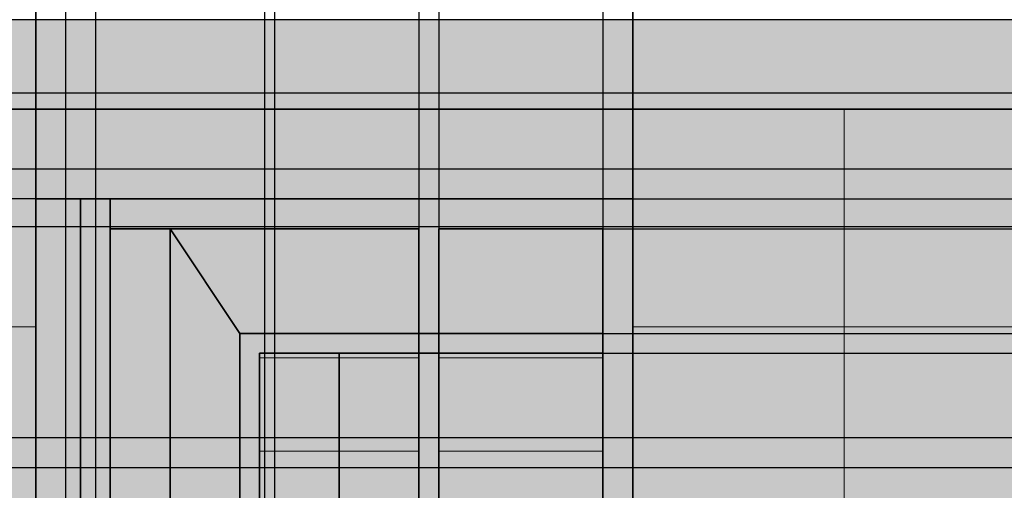
# Model space of a CAD drawing. Units: inches. Extents: x 148 to 1080, y 89 to 707.
# Tile 5 of 12: x 272 to 470, y 273 to 368. Entities that reach past the tile are written whole.
import ezdxf

# ---------------------------------------------------------------- set-up
doc = ezdxf.new("R2010")
doc.units = ezdxf.units.IN
doc.header["$MEASUREMENT"] = 0
for name, color, linetype, lineweight in [('A-ANNO-DIMS', 2, 'Continuous', 18), ('A-ELEV', 7, 'Continuous', 35), ('A-ELEV-PATT', 8, 'Continuous', 13)]:
    doc.layers.add(name, color=color, linetype=linetype, lineweight=lineweight)
doc.styles.get("Standard").update_dxf_attribs({"font": 'arial.ttf'})
doc.dimstyles.get("Standard").update_dxf_attribs({"dimtxt": 6, "dimasz": 0.18, "dimexe": 0.18, "dimexo": 0.0625, "dimgap": 0.09, "dimtad": 0, "dimtih": 1, "dimtoh": 1, "dimdec": 0, "dimzin": 0, "dimdsep": 46, "dimlunit": 3, "dimtxsty": 'Standard', "dimcen": 0.09, "dimadec": 0, "dimazin": 0, "dimtfac": 1, "dimtdec": 0, "dimtofl": 0, "dimtmove": 0, "dimatfit": 3, "dimfxl": 1, "dimtolj": 1, "dimtzin": 0, "dimarcsym": 0})

# ---------------------------------------------------------------- blocks, each defined once
blk = doc.blocks.new('*D1')
at = {"layer": 'A-ANNO-DIMS', "color": 0, "lineweight": -2, "transparency": 16777216}
for p, q in [((215.02, 662.01), (215.02, 703.28)), ((215.2, 703.1), (604.32, 703.1)), ((1006.77, 703.1), (617.65, 703.1)), ((1006.95, 338.01), (1006.95, 703.28))]:
    blk.add_line(p, q, dxfattribs=at)
at = {"layer": 'A-ANNO-DIMS', "color": 0, "transparency": 16777216}
for points in [[(215.2, 703.13), (215.2, 703.07), (215.02, 703.1)], [(1006.77, 703.13), (1006.77, 703.07), (1006.95, 703.1)]]:
    blk.add_solid(points, dxfattribs=at)
at = {"layer": 'Defpoints', "color": 0, "transparency": 16777216}
for p in [(1006.95, 703.1), (215.02, 661.95), (1006.95, 337.95)]:
    blk.add_point(p, dxfattribs=at)
at = {"layer": 'A-ANNO-DIMS', "color": 0, "transparency": 16777216, "insert": (610.98, 703.1), "char_height": 6, "attachment_point": 5}
blk.add_mtext('\\A1;792', dxfattribs=at)
blk = doc.blocks.new('*D27')
at = {"layer": 'A-ANNO-DIMS', "color": 0, "lineweight": -2, "transparency": 16777216}
for p, q in [((275.02, 332.01), (275.02, 703.28)), ((275.2, 703.1), (328.59, 703.1)), ((394.84, 703.1), (341.45, 703.1)), ((395.02, 332.01), (395.02, 703.28))]:
    blk.add_line(p, q, dxfattribs=at)
at = {"layer": 'A-ANNO-DIMS', "color": 0, "transparency": 16777216}
for points in [[(275.2, 703.13), (275.2, 703.07), (275.02, 703.1)], [(394.84, 703.13), (394.84, 703.07), (395.02, 703.1)]]:
    blk.add_solid(points, dxfattribs=at)
at = {"layer": 'Defpoints', "color": 0, "transparency": 16777216}
for p in [(395.02, 703.1), (275.02, 331.95), (395.02, 331.95)]:
    blk.add_point(p, dxfattribs=at)
at = {"layer": 'A-ANNO-DIMS', "color": 0, "transparency": 16777216, "insert": (335.02, 703.1), "char_height": 6, "attachment_point": 5}
blk.add_mtext('\\A1;120', dxfattribs=at)
blk = doc.blocks.new('*D28')
at = {"layer": 'A-ANNO-DIMS', "color": 0, "lineweight": -2, "transparency": 16777216}
for p, q in [((274.96, 331.95), (160.42, 331.95)), ((160.6, 331.77), (160.6, 251.1)), ((160.6, 164.13), (160.6, 244.79)), ((274.96, 163.95), (160.42, 163.95))]:
    blk.add_line(p, q, dxfattribs=at)
at = {"layer": 'A-ANNO-DIMS', "color": 0, "transparency": 16777216}
for points in [[(160.57, 331.77), (160.63, 331.77), (160.6, 331.95)], [(160.57, 164.13), (160.63, 164.13), (160.6, 163.95)]]:
    blk.add_solid(points, dxfattribs=at)
at = {"layer": 'Defpoints', "color": 0, "transparency": 16777216}
for p in [(160.6, 331.95), (275.02, 331.95), (275.02, 163.95)]:
    blk.add_point(p, dxfattribs=at)
at = {"layer": 'A-ANNO-DIMS', "color": 0, "transparency": 16777216, "insert": (160.6, 247.95), "char_height": 6, "attachment_point": 5}
blk.add_mtext('\\A1;168', dxfattribs=at)
blk = doc.blocks.new('*D34')
at = {"layer": 'A-ANNO-DIMS', "color": 0, "lineweight": -2, "transparency": 16777216}
for p, q in [((574.96, 283.95), (160.42, 283.95)), ((160.6, 283.77), (160.6, 212.1)), ((160.6, 134.13), (160.6, 205.79)), ((574.96, 133.95), (160.42, 133.95))]:
    blk.add_line(p, q, dxfattribs=at)
at = {"layer": 'A-ANNO-DIMS', "color": 0, "transparency": 16777216}
for points in [[(160.57, 283.77), (160.63, 283.77), (160.6, 283.95)], [(160.57, 134.13), (160.63, 134.13), (160.6, 133.95)]]:
    blk.add_solid(points, dxfattribs=at)
at = {"layer": 'Defpoints', "color": 0, "transparency": 16777216}
for p in [(575.02, 283.95), (160.6, 133.95), (575.02, 133.95)]:
    blk.add_point(p, dxfattribs=at)
at = {"layer": 'A-ANNO-DIMS', "color": 0, "transparency": 16777216, "insert": (160.6, 208.95), "char_height": 6, "attachment_point": 5}
blk.add_mtext('\\A1;150', dxfattribs=at)
blk = doc.blocks.new('*D39')
at = {"layer": 'A-ANNO-DIMS', "color": 0, "lineweight": -2, "transparency": 16777216}
for p, q in [((946.89, 337.95), (160.42, 337.95)), ((160.6, 337.77), (160.6, 311.1)), ((160.6, 278.13), (160.6, 304.79)), ((946.89, 277.95), (160.42, 277.95))]:
    blk.add_line(p, q, dxfattribs=at)
at = {"layer": 'A-ANNO-DIMS', "color": 0, "transparency": 16777216}
for points in [[(160.57, 337.77), (160.63, 337.77), (160.6, 337.95)], [(160.57, 278.13), (160.63, 278.13), (160.6, 277.95)]]:
    blk.add_solid(points, dxfattribs=at)
at = {"layer": 'Defpoints', "color": 0, "transparency": 16777216}
for p in [(160.6, 337.95), (946.95, 337.95), (946.95, 277.95)]:
    blk.add_point(p, dxfattribs=at)
at = {"layer": 'A-ANNO-DIMS', "color": 0, "transparency": 16777216, "insert": (160.6, 307.95), "char_height": 6, "attachment_point": 5}
blk.add_mtext('\\A1;60', dxfattribs=at)
blk = doc.blocks.new('*D42')
at = {"layer": 'A-ANNO-DIMS', "color": 0, "lineweight": -2, "transparency": 16777216}
for p, q in [((772.96, 367.95), (160.42, 367.95)), ((160.6, 367.77), (160.6, 350.31)), ((160.6, 326.54), (160.6, 344)), ((718.96, 326.36), (160.42, 326.36))]:
    blk.add_line(p, q, dxfattribs=at)
at = {"layer": 'A-ANNO-DIMS', "color": 0, "transparency": 16777216}
for points in [[(160.57, 367.77), (160.63, 367.77), (160.6, 367.95)], [(160.57, 326.54), (160.63, 326.54), (160.6, 326.36)]]:
    blk.add_solid(points, dxfattribs=at)
at = {"layer": 'Defpoints', "color": 0, "transparency": 16777216}
for p in [(773.02, 367.95), (160.6, 326.36), (719.02, 326.36)]:
    blk.add_point(p, dxfattribs=at)
at = {"layer": 'A-ANNO-DIMS', "color": 0, "transparency": 16777216, "insert": (160.6, 347.16), "char_height": 6, "attachment_point": 5}
blk.add_mtext('\\A1;41.584', dxfattribs=at)
blk = doc.blocks.new('*D49')
at = {"layer": 'A-ANNO-DIMS', "color": 0, "lineweight": -2, "transparency": 16777216}
for p, q in [((628.11, 353.2), (160.42, 353.2)), ((160.6, 353.02), (160.6, 348.73)), ((160.6, 338.13), (160.6, 342.42)), ((682.96, 337.95), (160.42, 337.95))]:
    blk.add_line(p, q, dxfattribs=at)
at = {"layer": 'A-ANNO-DIMS', "color": 0, "transparency": 16777216}
for points in [[(160.57, 353.02), (160.63, 353.02), (160.6, 353.2)], [(160.57, 338.13), (160.63, 338.13), (160.6, 337.95)]]:
    blk.add_solid(points, dxfattribs=at)
at = {"layer": 'Defpoints', "color": 0, "transparency": 16777216}
for p in [(628.17, 353.2), (160.6, 337.95), (683.02, 337.95)]:
    blk.add_point(p, dxfattribs=at)
at = {"layer": 'A-ANNO-DIMS', "color": 0, "transparency": 16777216, "insert": (160.6, 345.57), "char_height": 6, "attachment_point": 5}
blk.add_mtext('\\A1;15.248', dxfattribs=at)
blk = doc.blocks.new('*D76')
at = {"layer": 'A-ANNO-DIMS', "color": 0, "lineweight": -2, "transparency": 16777216}
for p, q in [((389.08, 300.95), (1064.5, 300.95)), ((1064.32, 300.77), (1064.32, 286.06)), ((1064.32, 265.05), (1064.32, 279.75)), ((389.08, 264.87), (1064.5, 264.87))]:
    blk.add_line(p, q, dxfattribs=at)
at = {"layer": 'A-ANNO-DIMS', "color": 0, "transparency": 16777216}
for points in [[(1064.29, 300.77), (1064.35, 300.77), (1064.32, 300.95)], [(1064.29, 265.05), (1064.35, 265.05), (1064.32, 264.87)]]:
    blk.add_solid(points, dxfattribs=at)
at = {"layer": 'Defpoints', "color": 0, "transparency": 16777216}
for p in [(389.02, 300.95), (1064.32, 300.95), (389.02, 264.87)]:
    blk.add_point(p, dxfattribs=at)
at = {"layer": 'A-ANNO-DIMS', "color": 0, "transparency": 16777216, "insert": (1064.32, 282.91), "char_height": 6, "attachment_point": 5}
blk.add_mtext('\\A1;36.08', dxfattribs=at)
blk = doc.blocks.new('*D77')
at = {"layer": 'A-ANNO-DIMS', "color": 0, "lineweight": -2, "transparency": 16777216}
for p, q in [((389.08, 304.95), (1064.5, 304.95)), ((1064.32, 304.95), (1064.32, 305.13)), ((1064.32, 305.13), (1064.5, 305.13)), ((1064.32, 301.13), (1064.32, 304.77)), ((389.08, 300.95), (1064.5, 300.95))]:
    blk.add_line(p, q, dxfattribs=at)
at = {"layer": 'A-ANNO-DIMS', "color": 0, "transparency": 16777216}
for points in [[(1064.29, 304.77), (1064.35, 304.77), (1064.32, 304.95)], [(1064.29, 301.13), (1064.35, 301.13), (1064.32, 300.95)]]:
    blk.add_solid(points, dxfattribs=at)
at = {"layer": 'Defpoints', "color": 0, "transparency": 16777216}
for p in [(389.02, 304.95), (1064.32, 304.95), (389.02, 300.95)]:
    blk.add_point(p, dxfattribs=at)
at = {"layer": 'A-ANNO-DIMS', "color": 0, "transparency": 16777216, "insert": (1072.5, 305.13), "char_height": 6, "attachment_point": 5}
blk.add_mtext('\\A1;4.00', dxfattribs=at)
blk = doc.blocks.new('*D78')
at = {"layer": 'A-ANNO-DIMS', "color": 0, "lineweight": -2, "transparency": 16777216}
for p, q in [((389.08, 325.95), (1064.5, 325.95)), ((1064.32, 325.77), (1064.32, 318.6)), ((1064.32, 305.13), (1064.32, 312.29)), ((389.08, 304.95), (1064.5, 304.95))]:
    blk.add_line(p, q, dxfattribs=at)
at = {"layer": 'A-ANNO-DIMS', "color": 0, "transparency": 16777216}
for points in [[(1064.29, 325.77), (1064.35, 325.77), (1064.32, 325.95)], [(1064.29, 305.13), (1064.35, 305.13), (1064.32, 304.95)]]:
    blk.add_solid(points, dxfattribs=at)
at = {"layer": 'Defpoints', "color": 0, "transparency": 16777216}
for p in [(389.02, 325.95), (1064.32, 325.95), (389.02, 304.95)]:
    blk.add_point(p, dxfattribs=at)
at = {"layer": 'A-ANNO-DIMS', "color": 0, "transparency": 16777216, "insert": (1064.32, 315.45), "char_height": 6, "attachment_point": 5}
blk.add_mtext('\\A1;21.00', dxfattribs=at)
blk = doc.blocks.new('*D79')
at = {"layer": 'A-ANNO-DIMS', "color": 0, "lineweight": -2, "transparency": 16777216}
for p, q in [((395.08, 331.95), (1064.5, 331.95)), ((1064.32, 331.95), (1064.32, 332.13)), ((1064.32, 332.13), (1064.5, 332.13)), ((1064.32, 326.13), (1064.32, 331.77)), ((389.08, 325.95), (1064.5, 325.95))]:
    blk.add_line(p, q, dxfattribs=at)
at = {"layer": 'A-ANNO-DIMS', "color": 0, "transparency": 16777216}
for points in [[(1064.29, 331.77), (1064.35, 331.77), (1064.32, 331.95)], [(1064.29, 326.13), (1064.35, 326.13), (1064.32, 325.95)]]:
    blk.add_solid(points, dxfattribs=at)
at = {"layer": 'Defpoints', "color": 0, "transparency": 16777216}
for p in [(395.02, 331.95), (1064.32, 331.95), (389.02, 325.95)]:
    blk.add_point(p, dxfattribs=at)
at = {"layer": 'A-ANNO-DIMS', "color": 0, "transparency": 16777216, "insert": (1072.39, 332.13), "char_height": 6, "attachment_point": 5}
blk.add_mtext('\\A1;6.00', dxfattribs=at)
blk = doc.blocks.new('*D82')
at = {"layer": 'A-ANNO-DIMS', "color": 0, "lineweight": -2, "transparency": 16777216}
for p, q in [((275.02, 400.88), (275.02, 92.62)), ((281.02, 400.88), (281.02, 92.62)), ((275.2, 92.8), (280.84, 92.8)), ((281.02, 92.8), (281.2, 92.8))]:
    blk.add_line(p, q, dxfattribs=at)
at = {"layer": 'A-ANNO-DIMS', "color": 0, "transparency": 16777216}
for points in [[(275.2, 92.83), (275.2, 92.77), (275.02, 92.8)], [(280.84, 92.83), (280.84, 92.77), (281.02, 92.8)]]:
    blk.add_solid(points, dxfattribs=at)
at = {"layer": 'Defpoints', "color": 0, "transparency": 16777216}
for p in [(275.02, 400.95), (281.02, 400.95), (281.02, 92.8)]:
    blk.add_point(p, dxfattribs=at)
at = {"layer": 'A-ANNO-DIMS', "color": 0, "transparency": 16777216, "insert": (289.09, 92.8), "char_height": 6, "attachment_point": 5}
blk.add_mtext('\\A1;6.00', dxfattribs=at)
blk = doc.blocks.new('*D83')
at = {"layer": 'A-ANNO-DIMS', "color": 0, "lineweight": -2, "transparency": 16777216}
for p, q in [((281.02, 400.88), (281.02, 92.62)), ((287.02, 400.88), (287.02, 92.62)), ((281.2, 92.8), (286.84, 92.8)), ((287.02, 92.8), (287.2, 92.8))]:
    blk.add_line(p, q, dxfattribs=at)
at = {"layer": 'A-ANNO-DIMS', "color": 0, "transparency": 16777216}
for points in [[(281.2, 92.83), (281.2, 92.77), (281.02, 92.8)], [(286.84, 92.83), (286.84, 92.77), (287.02, 92.8)]]:
    blk.add_solid(points, dxfattribs=at)
at = {"layer": 'Defpoints', "color": 0, "transparency": 16777216}
for p in [(281.02, 400.95), (287.02, 400.95), (287.02, 92.8)]:
    blk.add_point(p, dxfattribs=at)
at = {"layer": 'A-ANNO-DIMS', "color": 0, "transparency": 16777216, "insert": (295.09, 92.8), "char_height": 6, "attachment_point": 5}
blk.add_mtext('\\A1;6.00', dxfattribs=at)
blk = doc.blocks.new('*D84')
at = {"layer": 'A-ANNO-DIMS', "color": 0, "lineweight": -2, "transparency": 16777216}
for p, q in [((321.02, 529.88), (321.02, 92.62)), ((287.02, 400.88), (287.02, 92.62)), ((287.2, 92.8), (293.82, 92.8)), ((320.84, 92.8), (314.22, 92.8))]:
    blk.add_line(p, q, dxfattribs=at)
at = {"layer": 'A-ANNO-DIMS', "color": 0, "transparency": 16777216}
for points in [[(287.2, 92.83), (287.2, 92.77), (287.02, 92.8)], [(320.84, 92.83), (320.84, 92.77), (321.02, 92.8)]]:
    blk.add_solid(points, dxfattribs=at)
at = {"layer": 'Defpoints', "color": 0, "transparency": 16777216}
for p in [(321.02, 529.95), (287.02, 400.95), (321.02, 92.8)]:
    blk.add_point(p, dxfattribs=at)
at = {"layer": 'A-ANNO-DIMS', "color": 0, "transparency": 16777216, "insert": (304.02, 92.8), "char_height": 6, "attachment_point": 5}
blk.add_mtext('\\A1;34.00', dxfattribs=at)
blk = doc.blocks.new('*D85')
at = {"layer": 'A-ANNO-DIMS', "color": 0, "lineweight": -2, "transparency": 16777216}
for p, q in [((321.02, 529.88), (321.02, 92.62)), ((323.02, 400.88), (323.02, 92.62)), ((321.2, 92.8), (322.84, 92.8)), ((323.02, 92.8), (323.2, 92.8))]:
    blk.add_line(p, q, dxfattribs=at)
at = {"layer": 'A-ANNO-DIMS', "color": 0, "transparency": 16777216}
for points in [[(321.2, 92.83), (321.2, 92.77), (321.02, 92.8)], [(322.84, 92.83), (322.84, 92.77), (323.02, 92.8)]]:
    blk.add_solid(points, dxfattribs=at)
at = {"layer": 'Defpoints', "color": 0, "transparency": 16777216}
for p in [(321.02, 529.95), (323.02, 400.95), (323.02, 92.8)]:
    blk.add_point(p, dxfattribs=at)
at = {"layer": 'A-ANNO-DIMS', "color": 0, "transparency": 16777216, "insert": (331.12, 92.8), "char_height": 6, "attachment_point": 5}
blk.add_mtext('\\A1;2.00', dxfattribs=at)
blk = doc.blocks.new('*D86')
at = {"layer": 'A-ANNO-DIMS', "color": 0, "lineweight": -2, "transparency": 16777216}
for p, q in [((323.02, 400.88), (323.02, 92.62)), ((352.02, 400.88), (352.02, 92.62)), ((323.2, 92.8), (327.27, 92.8)), ((351.84, 92.8), (347.77, 92.8))]:
    blk.add_line(p, q, dxfattribs=at)
at = {"layer": 'A-ANNO-DIMS', "color": 0, "transparency": 16777216}
for points in [[(323.2, 92.83), (323.2, 92.77), (323.02, 92.8)], [(351.84, 92.83), (351.84, 92.77), (352.02, 92.8)]]:
    blk.add_solid(points, dxfattribs=at)
at = {"layer": 'Defpoints', "color": 0, "transparency": 16777216}
for p in [(323.02, 400.95), (352.02, 400.95), (352.02, 92.8)]:
    blk.add_point(p, dxfattribs=at)
at = {"layer": 'A-ANNO-DIMS', "color": 0, "transparency": 16777216, "insert": (337.52, 92.8), "char_height": 6, "attachment_point": 5}
blk.add_mtext('\\A1;29.00', dxfattribs=at)
blk = doc.blocks.new('*D87')
at = {"layer": 'A-ANNO-DIMS', "color": 0, "lineweight": -2, "transparency": 16777216}
for p, q in [((352.02, 400.88), (352.02, 92.62)), ((356.02, 400.88), (356.02, 92.62)), ((352.2, 92.8), (355.84, 92.8)), ((356.02, 92.8), (356.2, 92.8))]:
    blk.add_line(p, q, dxfattribs=at)
at = {"layer": 'A-ANNO-DIMS', "color": 0, "transparency": 16777216}
for points in [[(352.2, 92.83), (352.2, 92.77), (352.02, 92.8)], [(355.84, 92.83), (355.84, 92.77), (356.02, 92.8)]]:
    blk.add_solid(points, dxfattribs=at)
at = {"layer": 'Defpoints', "color": 0, "transparency": 16777216}
for p in [(352.02, 400.95), (356.02, 400.95), (356.02, 92.8)]:
    blk.add_point(p, dxfattribs=at)
at = {"layer": 'A-ANNO-DIMS', "color": 0, "transparency": 16777216, "insert": (364.19, 92.8), "char_height": 6, "attachment_point": 5}
blk.add_mtext('\\A1;4.00', dxfattribs=at)
blk = doc.blocks.new('*D88')
at = {"layer": 'A-ANNO-DIMS', "color": 0, "lineweight": -2, "transparency": 16777216}
for p, q in [((356.02, 400.88), (356.02, 92.62)), ((389.02, 400.88), (389.02, 92.62)), ((356.2, 92.8), (362.32, 92.8)), ((388.84, 92.8), (382.72, 92.8))]:
    blk.add_line(p, q, dxfattribs=at)
at = {"layer": 'A-ANNO-DIMS', "color": 0, "transparency": 16777216}
for points in [[(356.2, 92.83), (356.2, 92.77), (356.02, 92.8)], [(388.84, 92.83), (388.84, 92.77), (389.02, 92.8)]]:
    blk.add_solid(points, dxfattribs=at)
at = {"layer": 'Defpoints', "color": 0, "transparency": 16777216}
for p in [(356.02, 400.95), (389.02, 400.95), (389.02, 92.8)]:
    blk.add_point(p, dxfattribs=at)
at = {"layer": 'A-ANNO-DIMS', "color": 0, "transparency": 16777216, "insert": (372.52, 92.8), "char_height": 6, "attachment_point": 5}
blk.add_mtext('\\A1;33.00', dxfattribs=at)
blk = doc.blocks.new('*D89')
at = {"layer": 'A-ANNO-DIMS', "color": 0, "lineweight": -2, "transparency": 16777216}
for p, q in [((389.02, 400.88), (389.02, 92.62)), ((395.02, 400.88), (395.02, 92.62)), ((389.2, 92.8), (394.84, 92.8)), ((395.02, 92.8), (395.2, 92.8))]:
    blk.add_line(p, q, dxfattribs=at)
at = {"layer": 'A-ANNO-DIMS', "color": 0, "transparency": 16777216}
for points in [[(389.2, 92.83), (389.2, 92.77), (389.02, 92.8)], [(394.84, 92.83), (394.84, 92.77), (395.02, 92.8)]]:
    blk.add_solid(points, dxfattribs=at)
at = {"layer": 'Defpoints', "color": 0, "transparency": 16777216}
for p in [(389.02, 400.95), (395.02, 400.95), (395.02, 92.8)]:
    blk.add_point(p, dxfattribs=at)
at = {"layer": 'A-ANNO-DIMS', "color": 0, "transparency": 16777216, "insert": (403.09, 92.8), "char_height": 6, "attachment_point": 5}
blk.add_mtext('\\A1;6.00', dxfattribs=at)

msp = doc.modelspace()

# ---------------------------------------------------------------- hatches: boundary and pattern name
at = {"layer": 'A-ELEV-PATT'}
h = msp.add_hatch(color=256, dxfattribs=at)
h.dxf.hatch_style = 1
h.paths.add_polyline_path([(622.6005, 631.9474), (611.0199, 631.9474), (215.0199, 631.9474), (251.0199, 542.9352), (251.0199, 601.9474), (527.0199, 601.9474), (527.0199, 541.9474), (598.6005, 541.9474)])
h.paths.add_polyline_path([(558.5775, 608.9493, -1), (552.5775, 608.9493, -1)], flags=16)
h.paths.add_polyline_path([(586.7589, 556.0652, -1), (580.7589, 556.0652, -1)], flags=16)
h.paths.add_polyline_path([(635.0199, 631.9474), (622.6005, 631.9474), (598.6005, 541.9474), (611.0199, 541.9474)])
h.paths.add_polyline_path([(773.0199, 367.9474), (215.0199, 367.9474), (251.0199, 337.9474), (251.0199, 349.9474), (527.0199, 349.9474), (527.0199, 337.9474), (734.0628, 337.9474)])
h.paths.add_polyline_path([(631.1736, 353.1958, -1), (625.1736, 353.1958, -1)], flags=16)
h.paths.add_polyline_path([(729.9419, 354.8591, -1), (723.9419, 354.8591, -1)], flags=16)
h = msp.add_hatch(color=256, dxfattribs=at)
h.dxf.hatch_style = 1
h.paths.add_polyline_path([(395.0199, 349.9474), (275.0199, 349.9474), (275.0199, 331.9474), (395.0199, 331.9474)])
h.paths.add_polyline_path([(284.0199, 331.9474), (275.0199, 331.9474), (275.0199, 163.9474), (284.0199, 163.9474)])
h.paths.add_polyline_path([(395.0199, 601.9474), (251.0199, 601.9474), (251.0199, 589.9474), (395.0199, 589.9474)])
h = msp.add_hatch(color=256, dxfattribs=at)
h.dxf.hatch_style = 1
h.paths.add_polyline_path([(527.0199, 349.9474), (395.0199, 349.9474), (395.0199, 271.2774), (527.0199, 272.3839)])
h.paths.add_polyline_path([(275.0199, 349.9474), (251.0199, 349.9474), (251.0199, 270.0704), (275.0199, 270.2716)])
h.paths.add_polyline_path([(743.0199, 337.9474), (734.0628, 337.9474), (719.0199, 326.3632), (719.0199, 277.9474), (743.0199, 277.9474)])
h.paths.add_polyline_path([(743.0199, 277.9474), (719.0199, 277.9474), (719.0199, 133.9474), (743.0199, 133.9474)])
h.paths.add_polyline_path([(734.0628, 337.9474), (719.0199, 337.9474), (719.0199, 326.3632)])
h = msp.add_hatch(dxfattribs=at)
h.set_pattern_fill('ANSI37', color=256, scale=350, angle=135)
h.paths.add_polyline_path([(527.0199, 349.9474), (395.0199, 349.9474), (395.0199, 163.9474), (275.0199, 163.9474), (275.0199, 349.9474), (251.0199, 349.9474), (251.0199, 133.9474), (527.0199, 133.9474)])
h = msp.add_hatch(color=256, dxfattribs=at)
h.dxf.hatch_style = 1
h.paths.add_polyline_path([(290.0199, 331.9474), (284.0199, 331.9474), (284.0199, 163.9474), (395.0199, 163.9474), (395.0199, 331.9474), (290.0199, 331.9474), (290.0199, 325.9474), (352.0199, 325.9474), (352.0199, 304.9474), (356.0199, 304.9474), (356.0199, 325.9474), (389.0199, 325.9474), (389.0199, 169.9474), (290.0199, 169.9474)])
h.paths.add_polyline_path([(356.0199, 300.9474), (352.0199, 300.9474), (352.0199, 169.9474), (356.0199, 169.9474)], flags=17)
h.paths.add_polyline_path([(356.0199, 304.9474), (352.0199, 304.9474), (352.0199, 300.9474), (356.0199, 300.9474)], flags=17)
h = msp.add_hatch(color=256, dxfattribs=at)
h.dxf.hatch_style = 1
h.paths.add_polyline_path([(389.0199, 300.9474), (356.0199, 300.9474), (356.0199, 264.8696), (389.0199, 264.8696)])
h.paths.add_polyline_path([(389.0199, 325.9474), (356.0199, 325.9474), (356.0199, 304.9474), (389.0199, 304.9474)])
h.paths.add_polyline_path([(352.0199, 325.9474), (302.0199, 325.9474), (316.0199, 304.9474), (352.0199, 304.9474)])
h.paths.add_polyline_path([(316.0199, 304.9474), (302.0199, 325.9474), (302.0199, 169.9474), (316.0199, 169.9474)])
h.paths.add_polyline_path([(302.0199, 325.9474), (290.0199, 325.9474), (290.0199, 222.3199), (302.0199, 206.8913)])
h.paths.add_polyline_path([(320.0199, 300.9474), (352.0199, 300.9474), (352.0199, 304.9474), (316.0199, 304.9474), (316.0199, 169.9474), (320.0199, 169.9474)])
h.paths.add_polyline_path([(336.0199, 300.9474), (320.0199, 300.9474), (320.0199, 264.8696), (336.0199, 264.8696)], flags=17)
h.paths.add_polyline_path([(352.0199, 300.9474), (336.0199, 300.9474), (336.0199, 264.8696), (352.0199, 264.8696)])
h.paths.add_polyline_path([(389.0199, 304.9474), (356.0199, 304.9474), (356.0199, 300.9474), (389.0199, 300.9474)])
h.paths.add_polyline_path([(389.0199, 192.8696), (356.0199, 192.8696), (356.0199, 169.9474), (389.0199, 169.9474)])
h.paths.add_polyline_path([(389.0199, 216.8696), (356.0199, 216.8696), (356.0199, 192.8696), (389.0199, 192.8696)])
h.paths.add_polyline_path([(389.0199, 240.8696), (356.0199, 240.8696), (356.0199, 216.8696), (389.0199, 216.8696)])
h.paths.add_polyline_path([(389.0199, 264.8696), (356.0199, 264.8696), (356.0199, 240.8696), (389.0199, 240.8696)])
h.paths.add_polyline_path([(352.0199, 264.8696), (336.0199, 264.8696), (336.0199, 240.8696), (352.0199, 240.8696)])
h.paths.add_polyline_path([(336.0199, 264.8696), (320.0199, 264.8696), (320.0199, 240.8696), (336.0199, 240.8696)], flags=17)
h.paths.add_polyline_path([(336.0199, 240.8696), (320.0199, 240.8696), (320.0199, 216.8696), (336.0199, 216.8696)], flags=17)
h.paths.add_polyline_path([(352.0199, 240.8696), (336.0199, 240.8696), (336.0199, 216.8696), (352.0199, 216.8696)])
h.paths.add_polyline_path([(352.0199, 216.8696), (336.0199, 216.8696), (336.0199, 192.8696), (352.0199, 192.8696)])
h.paths.add_polyline_path([(336.0199, 216.8696), (320.0199, 216.8696), (320.0199, 192.8696), (336.0199, 192.8696)], flags=17)
h.paths.add_polyline_path([(336.0199, 192.8696), (320.0199, 192.8696), (320.0199, 169.9474), (336.0199, 169.9474)], flags=17)
h.paths.add_polyline_path([(352.0199, 192.8696), (336.0199, 192.8696), (336.0199, 169.9474), (352.0199, 169.9474)])
h = msp.add_hatch(dxfattribs=at)
h.set_pattern_fill('ANSI31', color=256, scale=150, angle=135)
h.paths.add_polyline_path([(389.0199, 192.8696), (356.0199, 192.8696), (356.0199, 169.9474), (389.0199, 169.9474)])
h.paths.add_polyline_path([(389.0199, 240.8696), (356.0199, 240.8696), (356.0199, 216.8696), (389.0199, 216.8696)])
h.paths.add_polyline_path([(389.0199, 216.8696), (356.0199, 216.8696), (356.0199, 192.8696), (389.0199, 192.8696)])
h.paths.add_polyline_path([(389.0199, 264.8696), (356.0199, 264.8696), (356.0199, 240.8696), (389.0199, 240.8696)])
h.paths.add_polyline_path([(389.0199, 300.9474), (356.0199, 300.9474), (356.0199, 264.8696), (389.0199, 264.8696)])
h.paths.add_polyline_path([(352.0199, 300.9474), (336.0199, 300.9474), (336.0199, 264.8696), (352.0199, 264.8696)])
h.paths.add_polyline_path([(336.0199, 300.9474), (320.0199, 300.9474), (320.0199, 264.8696), (336.0199, 264.8696)])
h.paths.add_polyline_path([(336.0199, 264.8696), (320.0199, 264.8696), (320.0199, 240.8696), (336.0199, 240.8696)])
h.paths.add_polyline_path([(352.0199, 264.8696), (336.0199, 264.8696), (336.0199, 240.8696), (352.0199, 240.8696)])
h.paths.add_polyline_path([(336.0199, 240.8696), (320.0199, 240.8696), (320.0199, 216.8696), (336.0199, 216.8696)])
h.paths.add_polyline_path([(352.0199, 240.8696), (336.0199, 240.8696), (336.0199, 216.8696), (352.0199, 216.8696)])
h.paths.add_polyline_path([(336.0199, 216.8696), (320.0199, 216.8696), (320.0199, 192.8696), (336.0199, 192.8696)])
h.paths.add_polyline_path([(352.0199, 216.8696), (336.0199, 216.8696), (336.0199, 192.8696), (352.0199, 192.8696)])
h.paths.add_polyline_path([(336.0199, 192.8696), (320.0199, 192.8696), (320.0199, 169.9474), (336.0199, 169.9474)])
h.paths.add_polyline_path([(352.0199, 192.8696), (336.0199, 192.8696), (336.0199, 169.9474), (352.0199, 169.9474)])

# ---------------------------------------------------------------- linework, layer by layer
at = {"layer": 'A-ELEV'}
for p, q in [((251.0199, 349.9474), (527.0199, 349.9474)), ((275.0199, 163.9474), (275.0199, 349.9474)), ((395.0199, 163.9474), (395.0199, 349.9474)), ((275.0199, 331.9474), (395.0199, 331.9474)), ((284.0199, 163.9474), (284.0199, 331.9474)), ((290.0199, 169.9474), (290.0199, 331.9474)), ((290.0199, 325.9474), (352.0199, 325.9474)), ((302.0199, 169.9474), (302.0199, 325.9474)), ((302.0199, 325.9474), (316.0199, 304.9474)), ((352.0199, 169.9474), (352.0199, 325.9474)), ((356.0199, 169.9474), (356.0199, 325.9474)), ((356.0199, 325.9474), (389.0199, 325.9474)), ((389.0199, 169.9474), (389.0199, 325.9474)), ((316.0199, 304.9474), (389.0199, 304.9474)), ((316.0199, 169.9474), (316.0199, 304.9474)), ((320.0199, 169.9474), (320.0199, 300.9474)), ((320.0199, 300.9474), (389.0199, 300.9474)), ((336.0199, 169.9474), (336.0199, 300.9474))]:
    msp.add_line(p, q, dxfattribs=at)

# ---------------------------------------------------------------- dimensions: what is measured, and where the dimension line sits
at = {"layer": 'A-ANNO-DIMS'}
for base, p1, p2, override, picture, middle in [((1006.9492, 703.0974), (215.0199, 661.9474), (1006.9492, 337.9474), {"dimdec": 0, "dimlfac": 1, "dimrnd": 0, "dimzin": 0, "dimdsep": 46, "dimlunit": 2}, '*D1', (610.9845, 703.0974)), ((395.0199, 703.0974), (275.0199, 331.9474), (395.0199, 331.9474), {"dimdec": 0, "dimlfac": 1, "dimrnd": 0, "dimzin": 0, "dimdsep": 46, "dimlunit": 2}, '*D27', (335.0199, 703.0974)), ((321.0199, 92.7974), (287.0199, 400.9474), (321.0199, 529.9474), {"dimdec": 2, "dimlfac": 1, "dimrnd": 0, "dimzin": 0, "dimdsep": 46, "dimlunit": 2}, '*D84', (304.0199, 92.7974)), ((323.0199, 92.7974), (321.0199, 529.9474), (323.0199, 400.9474), {"dimdec": 2, "dimlfac": 1, "dimrnd": 0, "dimzin": 0, "dimdsep": 46, "dimlunit": 2}, '*D85', (331.1234, 92.7974)), ((281.0199, 92.7974), (275.0199, 400.9474), (281.0199, 400.9474), {"dimdec": 2, "dimlfac": 1, "dimrnd": 0, "dimzin": 0, "dimdsep": 46, "dimlunit": 2}, '*D82', (289.0886, 92.7974)), ((287.0199, 92.7974), (281.0199, 400.9474), (287.0199, 400.9474), {"dimdec": 2, "dimlfac": 1, "dimrnd": 0, "dimzin": 0, "dimdsep": 46, "dimlunit": 2}, '*D83', (295.0886, 92.7974)), ((352.0199, 92.7974), (323.0199, 400.9474), (352.0199, 400.9474), {"dimdec": 2, "dimlfac": 1, "dimrnd": 0, "dimzin": 0, "dimdsep": 46, "dimlunit": 2}, '*D86', (337.5199, 92.7974)), ((356.0199, 92.7974), (352.0199, 400.9474), (356.0199, 400.9474), {"dimdec": 2, "dimlfac": 1, "dimrnd": 0, "dimzin": 0, "dimdsep": 46, "dimlunit": 2}, '*D87', (364.193, 92.7974)), ((389.0199, 92.7974), (356.0199, 400.9474), (389.0199, 400.9474), {"dimdec": 2, "dimlfac": 1, "dimrnd": 0, "dimzin": 0, "dimdsep": 46, "dimlunit": 2}, '*D88', (372.5199, 92.7974)), ((395.0199, 92.7974), (389.0199, 400.9474), (395.0199, 400.9474), {"dimdec": 2, "dimlfac": 1, "dimrnd": 0, "dimzin": 0, "dimdsep": 46, "dimlunit": 2}, '*D89', (403.0886, 92.7974))]:
    dim = msp.add_linear_dim(base=base, p1=p1, p2=p2, dimstyle='Standard', override=override, dxfattribs=at)
    dim.commit()
    dim.dimension.update_dxf_attribs({"geometry": picture, "text_midpoint": middle})
for base, p1, p2, override, picture, middle in [((160.5992, 326.3632), (773.0199, 367.9474), (719.0199, 326.3632), {"dimdec": 3, "dimlfac": 1, "dimrnd": 0, "dimzin": 0, "dimdsep": 46, "dimlunit": 2}, '*D42', (160.5992, 347.1553)), ((160.5992, 337.9474), (628.1736, 353.1958), (683.0199, 337.9474), {"dimdec": 3, "dimlfac": 1, "dimrnd": 0, "dimzin": 0, "dimdsep": 46, "dimlunit": 2}, '*D49', (160.5992, 345.5716)), ((160.5992, 337.9474), (946.9492, 277.9474), (946.9492, 337.9474), {"dimdec": 0, "dimlfac": 1, "dimrnd": 0, "dimzin": 0, "dimdsep": 46, "dimlunit": 2}, '*D39', (160.5992, 307.9474)), ((1064.325, 331.9474), (389.0199, 325.9474), (395.0199, 331.9474), {"dimdec": 2, "dimlfac": 1, "dimrnd": 0, "dimzin": 0, "dimdsep": 46, "dimlunit": 2}, '*D79', (1072.3937, 332.1274)), ((160.5992, 331.9474), (275.0199, 163.9474), (275.0199, 331.9474), {"dimdec": 0, "dimlfac": 1, "dimrnd": 0, "dimzin": 0, "dimdsep": 46, "dimlunit": 2}, '*D28', (160.5992, 247.9474)), ((1064.325, 325.9474), (389.0199, 304.9474), (389.0199, 325.9474), {"dimdec": 2, "dimlfac": 1, "dimrnd": 0, "dimzin": 0, "dimdsep": 46, "dimlunit": 2}, '*D78', (1064.325, 315.4474)), ((1064.325, 304.9474), (389.0199, 300.9474), (389.0199, 304.9474), {"dimdec": 2, "dimlfac": 1, "dimrnd": 0, "dimzin": 0, "dimdsep": 46, "dimlunit": 2}, '*D77', (1072.4981, 305.1274)), ((1064.325, 300.9474), (389.0199, 264.8696), (389.0199, 300.9474), {"dimdec": 2, "dimlfac": 1, "dimrnd": 0, "dimzin": 0, "dimdsep": 46, "dimlunit": 2}, '*D76', (1064.325, 282.9085)), ((160.5992, 133.9474), (575.0199, 283.9474), (575.0199, 133.9474), {"dimdec": 0, "dimlfac": 1, "dimrnd": 0, "dimzin": 0, "dimdsep": 46, "dimlunit": 2}, '*D34', (160.5992, 208.9474))]:
    dim = msp.add_linear_dim(base=base, p1=p1, p2=p2, angle=90, dimstyle='Standard', override=override, dxfattribs=at)
    dim.commit()
    dim.dimension.update_dxf_attribs({"geometry": picture, "text_midpoint": middle})

doc.saveas('drawing.dxf')
